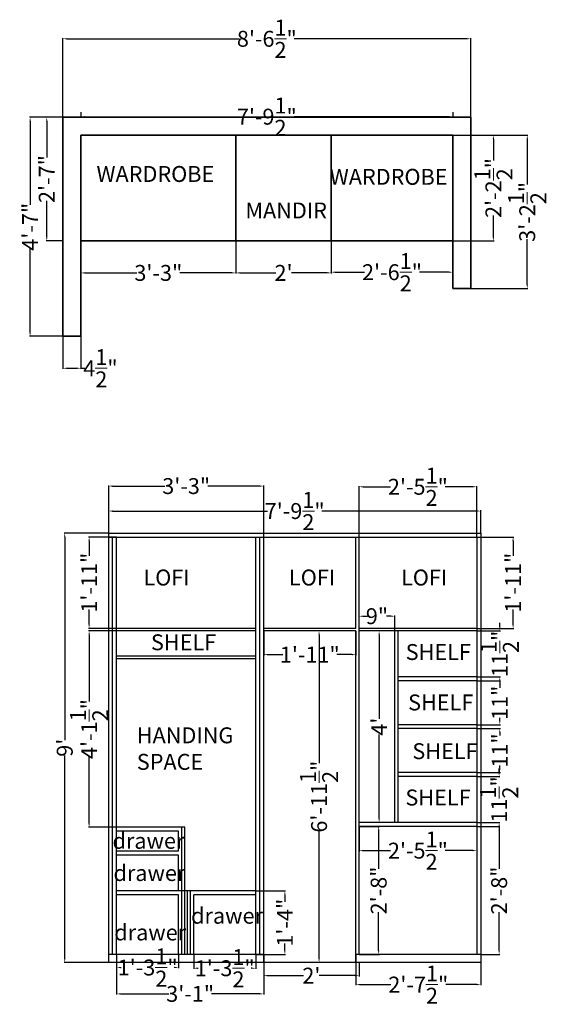
# Model space of a CAD drawing. Units: inches. Extents: x 198 to 331, y 201 to 449.
import ezdxf

# ---------------------------------------------------------------- set-up
doc = ezdxf.new("R2010")
doc.units = ezdxf.units.IN
doc.header["$MEASUREMENT"] = 0
for name, color, linetype, lineweight in [('A-ANNO-DIMS', 2, 'Continuous', 18), ('A-ANNO-TEXT', 3, 'Continuous', 18), ('A-ELEV', 7, 'Continuous', 25), ('A-FURN', 7, 'Continuous', 35)]:
    doc.layers.add(name, color=color, linetype=linetype, lineweight=lineweight)
doc.styles.get("Standard").update_dxf_attribs({"font": 'arial.ttf'})
doc.dimstyles.get("Standard").update_dxf_attribs({"dimtxt": 4, "dimasz": 1, "dimexe": 0.18, "dimexo": 0.0625, "dimgap": 0.09, "dimtad": 0, "dimdec": 1, "dimzin": 0, "dimdsep": 46, "dimlunit": 4, "dimtxsty": 'Standard', "dimcen": 0.09, "dimadec": 0, "dimazin": 0, "dimtfac": 1, "dimtdec": 1, "dimtofl": 0, "dimtmove": 0, "dimatfit": 3, "dimfxl": 1, "dimtolj": 1, "dimtzin": 0, "dimarcsym": 0})

# ---------------------------------------------------------------- blocks, each defined once
blk = doc.blocks.new('*D1')
at = {"layer": 'A-ANNO-DIMS', "color": 0, "lineweight": -2, "transparency": 16777216}
for p, q in [((307.47, 419.65), (317.79, 419.65)), ((317.61, 418.65), (317.61, 413.25)), ((317.61, 394.05), (317.61, 399.45)), ((307.47, 393.05), (317.79, 393.05))]:
    blk.add_line(p, q, dxfattribs=at)
at = {"layer": 'A-ANNO-DIMS', "color": 0, "transparency": 16777216}
for points in [[(317.44, 418.65), (317.77, 418.65), (317.61, 419.65)], [(317.44, 394.05), (317.77, 394.05), (317.61, 393.05)]]:
    blk.add_solid(points, dxfattribs=at)
at = {"layer": 'Defpoints', "color": 0, "transparency": 16777216}
for p in [(307.4, 419.65), (317.61, 419.65), (307.4, 393.05)]:
    blk.add_point(p, dxfattribs=at)
at = {"layer": 'A-ANNO-DIMS', "color": 0, "transparency": 16777216, "insert": (317.61, 406.35), "char_height": 4, "attachment_point": 5, "rotation": 90}
blk.add_mtext('\\A1;2\'-2{\\H1x;\\S1/2;}"', dxfattribs=at)
blk = doc.blocks.new('*D2')
at = {"layer": 'A-ANNO-DIMS', "color": 0, "lineweight": -2, "transparency": 16777216}
for p, q in [((276.8, 392.99), (276.8, 385)), ((307.4, 392.99), (307.4, 385)), ((277.8, 385.18), (285.21, 385.18)), ((306.4, 385.18), (299, 385.18))]:
    blk.add_line(p, q, dxfattribs=at)
at = {"layer": 'A-ANNO-DIMS', "color": 0, "transparency": 16777216}
for points in [[(277.8, 385.35), (277.8, 385.02), (276.8, 385.18)], [(306.4, 385.35), (306.4, 385.02), (307.4, 385.18)]]:
    blk.add_solid(points, dxfattribs=at)
at = {"layer": 'Defpoints', "color": 0, "transparency": 16777216}
for p in [(276.8, 393.05), (307.4, 393.05), (307.4, 385.18)]:
    blk.add_point(p, dxfattribs=at)
at = {"layer": 'A-ANNO-DIMS', "color": 0, "transparency": 16777216, "insert": (292.1, 385.18), "char_height": 4, "attachment_point": 5}
blk.add_mtext('\\A1;2\'-6{\\H1x;\\S1/2;}"', dxfattribs=at)
blk = doc.blocks.new('*D3')
at = {"layer": 'A-ANNO-DIMS', "color": 0, "lineweight": -2, "transparency": 16777216}
for p, q in [((252.8, 392.99), (252.8, 384.82)), ((276.8, 392.99), (276.8, 384.82)), ((253.8, 385), (262.84, 385)), ((275.8, 385), (266.77, 385))]:
    blk.add_line(p, q, dxfattribs=at)
at = {"layer": 'A-ANNO-DIMS', "color": 0, "transparency": 16777216}
for points in [[(253.8, 385.17), (253.8, 384.84), (252.8, 385)], [(275.8, 385.17), (275.8, 384.84), (276.8, 385)]]:
    blk.add_solid(points, dxfattribs=at)
at = {"layer": 'Defpoints', "color": 0, "transparency": 16777216}
for p in [(252.8, 393.05), (276.8, 393.05), (276.8, 385)]:
    blk.add_point(p, dxfattribs=at)
at = {"layer": 'A-ANNO-DIMS', "color": 0, "transparency": 16777216, "insert": (264.8, 385), "char_height": 4, "attachment_point": 5}
blk.add_mtext("\\A1;2'", dxfattribs=at)
blk = doc.blocks.new('*D4')
at = {"layer": 'A-ANNO-DIMS', "color": 0, "lineweight": -2, "transparency": 16777216}
for p, q in [((213.8, 392.99), (213.8, 384.82)), ((252.8, 392.99), (252.8, 384.82)), ((214.8, 385), (227.9, 385)), ((251.8, 385), (238.71, 385))]:
    blk.add_line(p, q, dxfattribs=at)
at = {"layer": 'A-ANNO-DIMS', "color": 0, "transparency": 16777216}
for points in [[(214.8, 385.17), (214.8, 384.84), (213.8, 385)], [(251.8, 385.17), (251.8, 384.84), (252.8, 385)]]:
    blk.add_solid(points, dxfattribs=at)
at = {"layer": 'Defpoints', "color": 0, "transparency": 16777216}
for p in [(213.8, 393.05), (252.8, 393.05), (252.8, 385)]:
    blk.add_point(p, dxfattribs=at)
at = {"layer": 'A-ANNO-DIMS', "color": 0, "transparency": 16777216, "insert": (233.3, 385), "char_height": 4, "attachment_point": 5}
blk.add_mtext('\\A1;3\'-3"', dxfattribs=at)
blk = doc.blocks.new('*D5')
at = {"layer": 'A-ANNO-DIMS', "color": 0, "lineweight": -2, "transparency": 16777216}
for p, q in [((213.8, 425.45), (213.8, 424.11)), ((214.8, 424.29), (253.76, 424.29)), ((306.4, 424.29), (267.45, 424.29)), ((307.4, 425.45), (307.4, 424.11))]:
    blk.add_line(p, q, dxfattribs=at)
at = {"layer": 'A-ANNO-DIMS', "color": 0, "transparency": 16777216}
for points in [[(214.8, 424.46), (214.8, 424.13), (213.8, 424.29)], [(306.4, 424.46), (306.4, 424.13), (307.4, 424.29)]]:
    blk.add_solid(points, dxfattribs=at)
at = {"layer": 'Defpoints', "color": 0, "transparency": 16777216}
for p in [(213.8, 425.51), (307.4, 425.51), (307.4, 424.29)]:
    blk.add_point(p, dxfattribs=at)
at = {"layer": 'A-ANNO-DIMS', "color": 0, "transparency": 16777216, "insert": (260.6, 424.29), "char_height": 4, "attachment_point": 5}
blk.add_mtext('\\A1;7\'-9{\\H1x;\\S1/2;}"', dxfattribs=at)
blk = doc.blocks.new('*D6')
at = {"layer": 'A-ANNO-DIMS', "color": 0, "lineweight": -2, "transparency": 16777216}
for p, q in [((222.81, 213.52), (222.81, 203.5)), ((259.81, 213.52), (259.81, 203.5)), ((223.81, 203.68), (235.91, 203.68)), ((258.81, 203.68), (246.72, 203.68))]:
    blk.add_line(p, q, dxfattribs=at)
at = {"layer": 'A-ANNO-DIMS', "color": 0, "transparency": 16777216}
for points in [[(223.81, 203.84), (223.81, 203.51), (222.81, 203.68)], [(258.81, 203.84), (258.81, 203.51), (259.81, 203.68)]]:
    blk.add_solid(points, dxfattribs=at)
at = {"layer": 'Defpoints', "color": 0, "transparency": 16777216}
for p in [(222.81, 213.58), (259.81, 213.58), (259.81, 203.68)]:
    blk.add_point(p, dxfattribs=at)
at = {"layer": 'A-ANNO-DIMS', "color": 0, "transparency": 16777216, "insert": (241.31, 203.68), "char_height": 4, "attachment_point": 5}
blk.add_mtext('\\A1;3\'-1"', dxfattribs=at)
blk = doc.blocks.new('*D7')
at = {"layer": 'A-ANNO-DIMS', "color": 0, "lineweight": -2, "transparency": 16777216}
for p, q in [((313.47, 318.58), (322.74, 318.58)), ((322.56, 317.58), (322.56, 313.85)), ((322.56, 296.58), (322.56, 300.31)), ((313.47, 295.58), (322.74, 295.58))]:
    blk.add_line(p, q, dxfattribs=at)
at = {"layer": 'A-ANNO-DIMS', "color": 0, "transparency": 16777216}
for points in [[(322.39, 317.58), (322.72, 317.58), (322.56, 318.58)], [(322.39, 296.58), (322.72, 296.58), (322.56, 295.58)]]:
    blk.add_solid(points, dxfattribs=at)
at = {"layer": 'Defpoints', "color": 0, "transparency": 16777216}
for p in [(313.41, 318.58), (313.41, 295.58), (322.56, 295.58)]:
    blk.add_point(p, dxfattribs=at)
at = {"layer": 'A-ANNO-DIMS', "color": 0, "transparency": 16777216, "insert": (322.56, 307.08), "char_height": 4, "attachment_point": 5, "rotation": 90}
blk.add_mtext('\\A1;1\'-11"', dxfattribs=at)
blk = doc.blocks.new('*D8')
at = {"layer": 'A-ANNO-DIMS', "color": 0, "lineweight": -2, "transparency": 16777216}
for p, q in [((313.47, 245.78), (319.23, 245.78)), ((319.05, 244.78), (319.05, 235.12)), ((319.05, 214.58), (319.05, 224.24)), ((314.47, 213.58), (319.23, 213.58))]:
    blk.add_line(p, q, dxfattribs=at)
at = {"layer": 'A-ANNO-DIMS', "color": 0, "transparency": 16777216}
for points in [[(318.88, 244.78), (319.21, 244.78), (319.05, 245.78)], [(318.88, 214.58), (319.21, 214.58), (319.05, 213.58)]]:
    blk.add_solid(points, dxfattribs=at)
at = {"layer": 'Defpoints', "color": 0, "transparency": 16777216}
for p in [(313.41, 245.78), (319.05, 245.78), (314.41, 213.58)]:
    blk.add_point(p, dxfattribs=at)
at = {"layer": 'A-ANNO-DIMS', "color": 0, "transparency": 16777216, "insert": (319.05, 229.68), "char_height": 4, "attachment_point": 5, "rotation": 90}
blk.add_mtext('\\A1;2\'-8"', dxfattribs=at)
blk = doc.blocks.new('*D9')
at = {"layer": 'A-ANNO-DIMS', "color": 0, "lineweight": -2, "transparency": 16777216}
for p, q in [((319.05, 259.38), (319.05, 260.38)), ((313.47, 258.38), (319.23, 258.38)), ((313.47, 246.78), (319.23, 246.78)), ((319.05, 245.78), (319.05, 244.78))]:
    blk.add_line(p, q, dxfattribs=at)
at = {"layer": 'A-ANNO-DIMS', "color": 0, "transparency": 16777216}
for points in [[(318.88, 259.38), (319.21, 259.38), (319.05, 258.38)], [(318.88, 245.78), (319.21, 245.78), (319.05, 246.78)]]:
    blk.add_solid(points, dxfattribs=at)
at = {"layer": 'Defpoints', "color": 0, "transparency": 16777216}
for p in [(313.41, 258.38), (313.41, 246.78), (319.05, 246.78)]:
    blk.add_point(p, dxfattribs=at)
at = {"layer": 'A-ANNO-DIMS', "color": 0, "transparency": 16777216, "insert": (319.05, 252.58), "char_height": 4, "attachment_point": 5, "rotation": 90}
blk.add_mtext('\\A1;11{\\H1x;\\S1/2;}"', dxfattribs=at)
blk = doc.blocks.new('*D10')
at = {"layer": 'A-ANNO-DIMS', "color": 0, "lineweight": -2, "transparency": 16777216}
for p, q in [((313.47, 270.38), (319.39, 270.38)), ((319.21, 269.38), (319.21, 268.63)), ((319.21, 260.38), (319.21, 261.13)), ((313.47, 259.38), (319.39, 259.38))]:
    blk.add_line(p, q, dxfattribs=at)
at = {"layer": 'A-ANNO-DIMS', "color": 0, "transparency": 16777216}
for points in [[(319.05, 269.38), (319.38, 269.38), (319.21, 270.38)], [(319.05, 260.38), (319.38, 260.38), (319.21, 259.38)]]:
    blk.add_solid(points, dxfattribs=at)
at = {"layer": 'Defpoints', "color": 0, "transparency": 16777216}
for p in [(313.41, 270.38), (313.41, 259.38), (319.21, 259.38)]:
    blk.add_point(p, dxfattribs=at)
at = {"layer": 'A-ANNO-DIMS', "color": 0, "transparency": 16777216, "insert": (319.21, 264.88), "char_height": 4, "attachment_point": 5, "rotation": 90}
blk.add_mtext('\\A1;11"', dxfattribs=at)
blk = doc.blocks.new('*D11')
at = {"layer": 'A-ANNO-DIMS', "color": 0, "lineweight": -2, "transparency": 16777216}
for p, q in [((313.47, 282.38), (319.39, 282.38)), ((319.21, 281.38), (319.21, 280.63)), ((319.21, 272.38), (319.21, 273.13)), ((313.47, 271.38), (319.39, 271.38))]:
    blk.add_line(p, q, dxfattribs=at)
at = {"layer": 'A-ANNO-DIMS', "color": 0, "transparency": 16777216}
for points in [[(319.05, 281.38), (319.38, 281.38), (319.21, 282.38)], [(319.05, 272.38), (319.38, 272.38), (319.21, 271.38)]]:
    blk.add_solid(points, dxfattribs=at)
at = {"layer": 'Defpoints', "color": 0, "transparency": 16777216}
for p in [(313.41, 282.38), (313.41, 271.38), (319.21, 271.38)]:
    blk.add_point(p, dxfattribs=at)
at = {"layer": 'A-ANNO-DIMS', "color": 0, "transparency": 16777216, "insert": (319.21, 276.88), "char_height": 4, "attachment_point": 5, "rotation": 90}
blk.add_mtext('\\A1;11"', dxfattribs=at)
blk = doc.blocks.new('*D12')
at = {"layer": 'A-ANNO-DIMS', "color": 0, "lineweight": -2, "transparency": 16777216}
for p, q in [((313.47, 294.98), (319.39, 294.98)), ((319.21, 295.98), (319.21, 296.98)), ((313.47, 283.38), (319.39, 283.38)), ((319.21, 282.38), (319.21, 281.38))]:
    blk.add_line(p, q, dxfattribs=at)
at = {"layer": 'A-ANNO-DIMS', "color": 0, "transparency": 16777216}
for points in [[(319.05, 295.98), (319.38, 295.98), (319.21, 294.98)], [(319.05, 282.38), (319.38, 282.38), (319.21, 283.38)]]:
    blk.add_solid(points, dxfattribs=at)
at = {"layer": 'Defpoints', "color": 0, "transparency": 16777216}
for p in [(313.41, 294.98), (313.41, 283.38), (319.21, 283.38)]:
    blk.add_point(p, dxfattribs=at)
at = {"layer": 'A-ANNO-DIMS', "color": 0, "transparency": 16777216, "insert": (319.21, 289.18), "char_height": 4, "attachment_point": 5, "rotation": 90}
blk.add_mtext('\\A1;11{\\H1x;\\S1/2;}"', dxfattribs=at)
blk = doc.blocks.new('*D13')
at = {"layer": 'A-ANNO-DIMS', "color": 0, "lineweight": -2, "transparency": 16777216}
for p, q in [((283.01, 213.52), (283.01, 205.83)), ((314.41, 213.52), (314.41, 205.83)), ((284.01, 206.01), (291.81, 206.01)), ((313.41, 206.01), (305.61, 206.01))]:
    blk.add_line(p, q, dxfattribs=at)
at = {"layer": 'A-ANNO-DIMS', "color": 0, "transparency": 16777216}
for points in [[(284.01, 206.17), (284.01, 205.84), (283.01, 206.01)], [(313.41, 206.17), (313.41, 205.84), (314.41, 206.01)]]:
    blk.add_solid(points, dxfattribs=at)
at = {"layer": 'Defpoints', "color": 0, "transparency": 16777216}
for p in [(283.01, 213.58), (314.41, 213.58), (283.01, 206.01)]:
    blk.add_point(p, dxfattribs=at)
at = {"layer": 'A-ANNO-DIMS', "color": 0, "transparency": 16777216, "insert": (298.71, 206.01), "char_height": 4, "attachment_point": 5}
blk.add_mtext('\\A1;2\'-7{\\H1x;\\S1/2;}"', dxfattribs=at)
blk = doc.blocks.new('*D14')
at = {"layer": 'A-ANNO-DIMS', "color": 0, "lineweight": -2, "transparency": 16777216}
for p, q in [((259.81, 211.52), (259.81, 208.08)), ((283.81, 211.52), (283.81, 208.08)), ((260.81, 208.26), (269.85, 208.26)), ((282.81, 208.26), (273.78, 208.26))]:
    blk.add_line(p, q, dxfattribs=at)
at = {"layer": 'A-ANNO-DIMS', "color": 0, "transparency": 16777216}
for points in [[(260.81, 208.43), (260.81, 208.09), (259.81, 208.26)], [(282.81, 208.43), (282.81, 208.09), (283.81, 208.26)]]:
    blk.add_solid(points, dxfattribs=at)
at = {"layer": 'Defpoints', "color": 0, "transparency": 16777216}
for p in [(259.81, 211.58), (283.81, 211.58), (283.81, 208.26)]:
    blk.add_point(p, dxfattribs=at)
at = {"layer": 'A-ANNO-DIMS', "color": 0, "transparency": 16777216, "insert": (271.81, 208.26), "char_height": 4, "attachment_point": 5}
blk.add_mtext("\\A1;2'", dxfattribs=at)
blk = doc.blocks.new('*D15')
at = {"layer": 'A-ANNO-DIMS', "color": 0, "lineweight": -2, "transparency": 16777216}
for p, q in [((222.81, 213.52), (222.81, 210.13)), ((238.41, 213.52), (238.41, 210.13)), ((223.81, 210.31), (223.93, 210.31)), ((237.41, 210.31), (237.29, 210.31))]:
    blk.add_line(p, q, dxfattribs=at)
at = {"layer": 'A-ANNO-DIMS', "color": 0, "transparency": 16777216}
for points in [[(223.81, 210.47), (223.81, 210.14), (222.81, 210.31)], [(237.41, 210.47), (237.41, 210.14), (238.41, 210.31)]]:
    blk.add_solid(points, dxfattribs=at)
at = {"layer": 'Defpoints', "color": 0, "transparency": 16777216}
for p in [(222.81, 213.58), (238.41, 213.58), (222.81, 210.31)]:
    blk.add_point(p, dxfattribs=at)
at = {"layer": 'A-ANNO-DIMS', "color": 0, "transparency": 16777216, "insert": (230.61, 210.31), "char_height": 4, "attachment_point": 5}
blk.add_mtext('\\A1;1\'-3{\\H1x;\\S1/2;}"', dxfattribs=at)
blk = doc.blocks.new('*D16')
at = {"layer": 'A-ANNO-DIMS', "color": 0, "lineweight": -2, "transparency": 16777216}
for p, q in [((242.21, 213.52), (242.21, 209.95)), ((257.81, 213.52), (257.81, 209.95)), ((243.21, 210.13), (243.33, 210.13)), ((256.81, 210.13), (256.69, 210.13))]:
    blk.add_line(p, q, dxfattribs=at)
at = {"layer": 'A-ANNO-DIMS', "color": 0, "transparency": 16777216}
for points in [[(243.21, 210.29), (243.21, 209.96), (242.21, 210.13)], [(256.81, 210.29), (256.81, 209.96), (257.81, 210.13)]]:
    blk.add_solid(points, dxfattribs=at)
at = {"layer": 'Defpoints', "color": 0, "transparency": 16777216}
for p in [(242.21, 213.58), (257.81, 213.58), (257.81, 210.13)]:
    blk.add_point(p, dxfattribs=at)
at = {"layer": 'A-ANNO-DIMS', "color": 0, "transparency": 16777216, "insert": (250.01, 210.13), "char_height": 4, "attachment_point": 5}
blk.add_mtext('\\A1;1\'-3{\\H1x;\\S1/2;}"', dxfattribs=at)
blk = doc.blocks.new('*D17')
at = {"layer": 'A-ANNO-DIMS', "color": 0, "lineweight": -2, "transparency": 16777216}
for p, q in [((257.87, 229.58), (265.32, 229.58)), ((265.14, 228.58), (265.14, 226.8)), ((265.14, 214.58), (265.14, 216.36)), ((257.87, 213.58), (265.32, 213.58))]:
    blk.add_line(p, q, dxfattribs=at)
at = {"layer": 'A-ANNO-DIMS', "color": 0, "transparency": 16777216}
for points in [[(264.98, 228.58), (265.31, 228.58), (265.14, 229.58)], [(264.98, 214.58), (265.31, 214.58), (265.14, 213.58)]]:
    blk.add_solid(points, dxfattribs=at)
at = {"layer": 'Defpoints', "color": 0, "transparency": 16777216}
for p in [(257.81, 229.58), (257.81, 213.58), (265.14, 213.58)]:
    blk.add_point(p, dxfattribs=at)
at = {"layer": 'A-ANNO-DIMS', "color": 0, "transparency": 16777216, "insert": (265.14, 221.58), "char_height": 4, "attachment_point": 5, "rotation": 90}
blk.add_mtext('\\A1;1\'-4"', dxfattribs=at)
blk = doc.blocks.new('*D18')
at = {"layer": 'A-ANNO-DIMS', "color": 0, "lineweight": -2, "transparency": 16777216}
for p, q in [((222.75, 294.98), (215.71, 294.98)), ((215.89, 293.98), (215.89, 277.22)), ((215.89, 246.58), (215.89, 263.33)), ((222.75, 245.58), (215.71, 245.58))]:
    blk.add_line(p, q, dxfattribs=at)
at = {"layer": 'A-ANNO-DIMS', "color": 0, "transparency": 16777216}
for points in [[(215.72, 293.98), (216.05, 293.98), (215.89, 294.98)], [(215.72, 246.58), (216.05, 246.58), (215.89, 245.58)]]:
    blk.add_solid(points, dxfattribs=at)
at = {"layer": 'Defpoints', "color": 0, "transparency": 16777216}
for p in [(215.89, 294.98), (222.81, 294.98), (222.81, 245.58)]:
    blk.add_point(p, dxfattribs=at)
at = {"layer": 'A-ANNO-DIMS', "color": 0, "transparency": 16777216, "insert": (215.89, 270.28), "char_height": 4, "attachment_point": 5, "rotation": 90}
blk.add_mtext('\\A1;4\'-1{\\H1x;\\S1/2;}"', dxfattribs=at)
blk = doc.blocks.new('*D19')
at = {"layer": 'A-ANNO-DIMS', "color": 0, "lineweight": -2, "transparency": 16777216}
for p, q in [((222.75, 318.58), (215.71, 318.58)), ((215.89, 317.58), (215.89, 313.85)), ((215.89, 296.58), (215.89, 300.31)), ((222.75, 295.58), (215.71, 295.58))]:
    blk.add_line(p, q, dxfattribs=at)
at = {"layer": 'A-ANNO-DIMS', "color": 0, "transparency": 16777216}
for points in [[(215.72, 317.58), (216.05, 317.58), (215.89, 318.58)], [(215.72, 296.58), (216.05, 296.58), (215.89, 295.58)]]:
    blk.add_solid(points, dxfattribs=at)
at = {"layer": 'Defpoints', "color": 0, "transparency": 16777216}
for p in [(215.89, 318.58), (222.81, 318.58), (222.81, 295.58)]:
    blk.add_point(p, dxfattribs=at)
at = {"layer": 'A-ANNO-DIMS', "color": 0, "transparency": 16777216, "insert": (215.89, 307.08), "char_height": 4, "attachment_point": 5, "rotation": 90}
blk.add_mtext('\\A1;1\'-11"', dxfattribs=at)
blk = doc.blocks.new('*D20')
at = {"layer": 'A-ANNO-DIMS', "color": 0, "lineweight": -2, "transparency": 16777216}
for p, q in [((220.81, 319.64), (220.81, 325.29)), ((221.81, 325.11), (260.76, 325.11)), ((313.41, 325.11), (274.46, 325.11)), ((314.41, 319.64), (314.41, 325.29))]:
    blk.add_line(p, q, dxfattribs=at)
at = {"layer": 'A-ANNO-DIMS', "color": 0, "transparency": 16777216}
for points in [[(221.81, 325.28), (221.81, 324.95), (220.81, 325.11)], [(313.41, 325.28), (313.41, 324.95), (314.41, 325.11)]]:
    blk.add_solid(points, dxfattribs=at)
at = {"layer": 'Defpoints', "color": 0, "transparency": 16777216}
for p in [(314.41, 325.11), (220.81, 319.58), (314.41, 319.58)]:
    blk.add_point(p, dxfattribs=at)
at = {"layer": 'A-ANNO-DIMS', "color": 0, "transparency": 16777216, "insert": (267.61, 325.11), "char_height": 4, "attachment_point": 5}
blk.add_mtext('\\A1;7\'-9{\\H1x;\\S1/2;}"', dxfattribs=at)
blk = doc.blocks.new('*D21')
at = {"layer": 'A-ANNO-DIMS', "color": 0, "lineweight": -2, "transparency": 16777216}
for p, q in [((220.75, 319.58), (209.57, 319.58)), ((209.75, 318.58), (209.75, 267.51)), ((209.75, 212.58), (209.75, 263.65)), ((220.75, 211.58), (209.57, 211.58))]:
    blk.add_line(p, q, dxfattribs=at)
at = {"layer": 'A-ANNO-DIMS', "color": 0, "transparency": 16777216}
for points in [[(209.59, 318.58), (209.92, 318.58), (209.75, 319.58)], [(209.59, 212.58), (209.92, 212.58), (209.75, 211.58)]]:
    blk.add_solid(points, dxfattribs=at)
at = {"layer": 'Defpoints', "color": 0, "transparency": 16777216}
for p in [(209.75, 319.58), (220.81, 319.58), (220.81, 211.58)]:
    blk.add_point(p, dxfattribs=at)
at = {"layer": 'A-ANNO-DIMS', "color": 0, "transparency": 16777216, "insert": (209.75, 265.58), "char_height": 4, "attachment_point": 5, "rotation": 90}
blk.add_mtext("\\A1;9'", dxfattribs=at)
blk = doc.blocks.new('*D22')
at = {"layer": 'A-ANNO-DIMS', "color": 0, "lineweight": -2, "transparency": 16777216}
for p, q in [((282.95, 294.98), (273.56, 294.98)), ((273.74, 293.98), (273.74, 261.71)), ((273.74, 212.58), (273.74, 244.85)), ((282.95, 211.58), (273.56, 211.58))]:
    blk.add_line(p, q, dxfattribs=at)
at = {"layer": 'A-ANNO-DIMS', "color": 0, "transparency": 16777216}
for points in [[(273.58, 293.98), (273.91, 293.98), (273.74, 294.98)], [(273.58, 212.58), (273.91, 212.58), (273.74, 211.58)]]:
    blk.add_solid(points, dxfattribs=at)
at = {"layer": 'Defpoints', "color": 0, "transparency": 16777216}
for p in [(273.74, 294.98), (283.01, 294.98), (283.01, 211.58)]:
    blk.add_point(p, dxfattribs=at)
at = {"layer": 'A-ANNO-DIMS', "color": 0, "transparency": 16777216, "insert": (273.74, 253.28), "char_height": 4, "attachment_point": 5, "rotation": 90}
blk.add_mtext('\\A1;6\'-11{\\H1x;\\S1/2;}"', dxfattribs=at)
blk = doc.blocks.new('*D23')
at = {"layer": 'A-ANNO-DIMS', "color": 0, "lineweight": -2, "transparency": 16777216}
for p, q in [((283.87, 245.78), (288.92, 245.78)), ((288.74, 244.78), (288.74, 235.12)), ((288.74, 214.58), (288.74, 224.24)), ((283.87, 213.58), (288.92, 213.58))]:
    blk.add_line(p, q, dxfattribs=at)
at = {"layer": 'A-ANNO-DIMS', "color": 0, "transparency": 16777216}
for points in [[(288.58, 244.78), (288.91, 244.78), (288.74, 245.78)], [(288.58, 214.58), (288.91, 214.58), (288.74, 213.58)]]:
    blk.add_solid(points, dxfattribs=at)
at = {"layer": 'Defpoints', "color": 0, "transparency": 16777216}
for p in [(283.81, 245.78), (283.81, 213.58), (288.74, 213.58)]:
    blk.add_point(p, dxfattribs=at)
at = {"layer": 'A-ANNO-DIMS', "color": 0, "transparency": 16777216, "insert": (288.74, 229.68), "char_height": 4, "attachment_point": 5, "rotation": 90}
blk.add_mtext('\\A1;2\'-8"', dxfattribs=at)
blk = doc.blocks.new('*D24')
at = {"layer": 'A-ANNO-DIMS', "color": 0, "lineweight": -2, "transparency": 16777216}
for p, q in [((283.81, 245.72), (283.81, 239.52)), ((313.41, 245.72), (313.41, 239.52)), ((284.81, 239.7), (291.71, 239.7)), ((312.41, 239.7), (305.51, 239.7))]:
    blk.add_line(p, q, dxfattribs=at)
at = {"layer": 'A-ANNO-DIMS', "color": 0, "transparency": 16777216}
for points in [[(284.81, 239.87), (284.81, 239.54), (283.81, 239.7)], [(312.41, 239.87), (312.41, 239.54), (313.41, 239.7)]]:
    blk.add_solid(points, dxfattribs=at)
at = {"layer": 'Defpoints', "color": 0, "transparency": 16777216}
for p in [(283.81, 245.78), (313.41, 245.78), (283.81, 239.7)]:
    blk.add_point(p, dxfattribs=at)
at = {"layer": 'A-ANNO-DIMS', "color": 0, "transparency": 16777216, "insert": (298.61, 239.7), "char_height": 4, "attachment_point": 5}
blk.add_mtext('\\A1;2\'-5{\\H1x;\\S1/2;}"', dxfattribs=at)
blk = doc.blocks.new('*D25')
at = {"layer": 'A-ANNO-DIMS', "color": 0, "lineweight": -2, "transparency": 16777216}
for p, q in [((259.81, 294.92), (259.81, 288.81)), ((283.01, 294.92), (283.01, 288.81)), ((260.81, 288.99), (264.64, 288.99)), ((282.01, 288.99), (278.18, 288.99))]:
    blk.add_line(p, q, dxfattribs=at)
at = {"layer": 'A-ANNO-DIMS', "color": 0, "transparency": 16777216}
for points in [[(260.81, 289.16), (260.81, 288.83), (259.81, 288.99)], [(282.01, 289.16), (282.01, 288.83), (283.01, 288.99)]]:
    blk.add_solid(points, dxfattribs=at)
at = {"layer": 'Defpoints', "color": 0, "transparency": 16777216}
for p in [(259.81, 294.98), (283.01, 294.98), (259.81, 288.99)]:
    blk.add_point(p, dxfattribs=at)
at = {"layer": 'A-ANNO-DIMS', "color": 0, "transparency": 16777216, "insert": (271.41, 288.99), "char_height": 4, "attachment_point": 5}
blk.add_mtext('\\A1;1\'-11"', dxfattribs=at)
blk = doc.blocks.new('*D26')
at = {"layer": 'A-ANNO-DIMS', "color": 0, "lineweight": -2, "transparency": 16777216}
for p, q in [((283.81, 295.04), (283.81, 298.84)), ((284.81, 298.66), (285.92, 298.66)), ((291.81, 298.66), (290.7, 298.66)), ((292.81, 295.04), (292.81, 298.84))]:
    blk.add_line(p, q, dxfattribs=at)
at = {"layer": 'A-ANNO-DIMS', "color": 0, "transparency": 16777216}
for points in [[(284.81, 298.83), (284.81, 298.49), (283.81, 298.66)], [(291.81, 298.83), (291.81, 298.49), (292.81, 298.66)]]:
    blk.add_solid(points, dxfattribs=at)
at = {"layer": 'Defpoints', "color": 0, "transparency": 16777216}
for p in [(292.81, 298.66), (283.81, 294.98), (292.81, 294.98)]:
    blk.add_point(p, dxfattribs=at)
at = {"layer": 'A-ANNO-DIMS', "color": 0, "transparency": 16777216, "insert": (288.31, 298.66), "char_height": 4, "attachment_point": 5}
blk.add_mtext('\\A1;9"', dxfattribs=at)
blk = doc.blocks.new('*D27')
at = {"layer": 'A-ANNO-DIMS', "color": 0, "lineweight": -2, "transparency": 16777216}
for p, q in [((292.75, 294.98), (288.68, 294.98)), ((288.86, 293.98), (288.86, 272.89)), ((288.86, 247.78), (288.86, 268.87)), ((292.75, 246.78), (288.68, 246.78))]:
    blk.add_line(p, q, dxfattribs=at)
at = {"layer": 'A-ANNO-DIMS', "color": 0, "transparency": 16777216}
for points in [[(288.7, 293.98), (289.03, 293.98), (288.86, 294.98)], [(288.7, 247.78), (289.03, 247.78), (288.86, 246.78)]]:
    blk.add_solid(points, dxfattribs=at)
at = {"layer": 'Defpoints', "color": 0, "transparency": 16777216}
for p in [(288.86, 294.98), (292.81, 294.98), (292.81, 246.78)]:
    blk.add_point(p, dxfattribs=at)
at = {"layer": 'A-ANNO-DIMS', "color": 0, "transparency": 16777216, "insert": (288.86, 270.88), "char_height": 4, "attachment_point": 5, "rotation": 90}
blk.add_mtext("\\A1;4'", dxfattribs=at)
blk = doc.blocks.new('*D28')
at = {"layer": 'A-ANNO-DIMS', "color": 0, "lineweight": -2, "transparency": 16777216}
for p, q in [((283.81, 318.64), (283.81, 331.39)), ((284.81, 331.21), (291.71, 331.21)), ((312.41, 331.21), (305.51, 331.21)), ((313.41, 318.64), (313.41, 331.39))]:
    blk.add_line(p, q, dxfattribs=at)
at = {"layer": 'A-ANNO-DIMS', "color": 0, "transparency": 16777216}
for points in [[(284.81, 331.37), (284.81, 331.04), (283.81, 331.21)], [(312.41, 331.37), (312.41, 331.04), (313.41, 331.21)]]:
    blk.add_solid(points, dxfattribs=at)
at = {"layer": 'Defpoints', "color": 0, "transparency": 16777216}
for p in [(283.81, 331.21), (283.81, 318.58), (313.41, 318.58)]:
    blk.add_point(p, dxfattribs=at)
at = {"layer": 'A-ANNO-DIMS', "color": 0, "transparency": 16777216, "insert": (298.61, 331.21), "char_height": 4, "attachment_point": 5}
blk.add_mtext('\\A1;2\'-5{\\H1x;\\S1/2;}"', dxfattribs=at)
blk = doc.blocks.new('*D29')
at = {"layer": 'A-ANNO-DIMS', "color": 0, "lineweight": -2, "transparency": 16777216}
for p, q in [((220.81, 318.64), (220.81, 331.57)), ((221.81, 331.39), (234.91, 331.39)), ((258.81, 331.39), (245.72, 331.39)), ((259.81, 318.64), (259.81, 331.57))]:
    blk.add_line(p, q, dxfattribs=at)
at = {"layer": 'A-ANNO-DIMS', "color": 0, "transparency": 16777216}
for points in [[(221.81, 331.55), (221.81, 331.22), (220.81, 331.39)], [(258.81, 331.55), (258.81, 331.22), (259.81, 331.39)]]:
    blk.add_solid(points, dxfattribs=at)
at = {"layer": 'Defpoints', "color": 0, "transparency": 16777216}
for p in [(259.81, 331.39), (220.81, 318.58), (259.81, 318.58)]:
    blk.add_point(p, dxfattribs=at)
at = {"layer": 'A-ANNO-DIMS', "color": 0, "transparency": 16777216, "insert": (240.31, 331.39), "char_height": 4, "attachment_point": 5}
blk.add_mtext('\\A1;3\'-3"', dxfattribs=at)
blk = doc.blocks.new('*D30')
at = {"layer": 'A-ANNO-DIMS', "color": 0, "lineweight": -2, "transparency": 16777216}
for p, q in [((209.3, 424.21), (209.3, 444.06)), ((210.3, 443.88), (253.74, 443.88)), ((310.9, 443.88), (267.47, 443.88)), ((311.9, 424.21), (311.9, 444.06))]:
    blk.add_line(p, q, dxfattribs=at)
at = {"layer": 'A-ANNO-DIMS', "color": 0, "transparency": 16777216}
for points in [[(210.3, 444.05), (210.3, 443.72), (209.3, 443.88)], [(310.9, 444.05), (310.9, 443.72), (311.9, 443.88)]]:
    blk.add_solid(points, dxfattribs=at)
at = {"layer": 'Defpoints', "color": 0, "transparency": 16777216}
for p in [(311.9, 443.88), (209.3, 424.15), (311.9, 424.15)]:
    blk.add_point(p, dxfattribs=at)
at = {"layer": 'A-ANNO-DIMS', "color": 0, "transparency": 16777216, "insert": (260.6, 443.88), "char_height": 4, "attachment_point": 5}
blk.add_mtext('\\A1;8\'-6{\\H1x;\\S1/2;}"', dxfattribs=at)
blk = doc.blocks.new('*D31')
at = {"layer": 'A-ANNO-DIMS', "color": 0, "lineweight": -2, "transparency": 16777216}
for p, q in [((209.24, 424.15), (205.05, 424.15)), ((205.23, 423.15), (205.23, 414.04)), ((205.23, 394.05), (205.23, 403.16)), ((209.24, 393.05), (205.05, 393.05))]:
    blk.add_line(p, q, dxfattribs=at)
at = {"layer": 'A-ANNO-DIMS', "color": 0, "transparency": 16777216}
for points in [[(205.07, 423.15), (205.4, 423.15), (205.23, 424.15)], [(205.07, 394.05), (205.4, 394.05), (205.23, 393.05)]]:
    blk.add_solid(points, dxfattribs=at)
at = {"layer": 'Defpoints', "color": 0, "transparency": 16777216}
for p in [(209.3, 424.15), (205.23, 393.05), (209.3, 393.05)]:
    blk.add_point(p, dxfattribs=at)
at = {"layer": 'A-ANNO-DIMS', "color": 0, "transparency": 16777216, "insert": (205.23, 408.6), "char_height": 4, "attachment_point": 5, "rotation": 90}
blk.add_mtext('\\A1;2\'-7"', dxfattribs=at)
blk = doc.blocks.new('*D32')
at = {"layer": 'A-ANNO-DIMS', "color": 0, "lineweight": -2, "transparency": 16777216}
for p, q in [((209.24, 424.15), (200.86, 424.15)), ((201.04, 423.15), (201.04, 402.09)), ((201.04, 370.05), (201.04, 391.11)), ((209.24, 369.05), (200.86, 369.05))]:
    blk.add_line(p, q, dxfattribs=at)
at = {"layer": 'A-ANNO-DIMS', "color": 0, "transparency": 16777216}
for points in [[(200.87, 423.15), (201.21, 423.15), (201.04, 424.15)], [(200.87, 370.05), (201.21, 370.05), (201.04, 369.05)]]:
    blk.add_solid(points, dxfattribs=at)
at = {"layer": 'Defpoints', "color": 0, "transparency": 16777216}
for p in [(209.3, 424.15), (201.04, 369.05), (209.3, 369.05)]:
    blk.add_point(p, dxfattribs=at)
at = {"layer": 'A-ANNO-DIMS', "color": 0, "transparency": 16777216, "insert": (201.04, 396.6), "char_height": 4, "attachment_point": 5, "rotation": 90}
blk.add_mtext('\\A1;4\'-7"', dxfattribs=at)
blk = doc.blocks.new('*D33')
at = {"layer": 'A-ANNO-DIMS', "color": 0, "lineweight": -2, "transparency": 16777216}
for p, q in [((209.3, 368.99), (209.3, 360.84)), ((213.8, 368.99), (213.8, 360.84)), ((210.3, 361.02), (212.8, 361.02)), ((213.8, 361.02), (214.8, 361.02))]:
    blk.add_line(p, q, dxfattribs=at)
at = {"layer": 'A-ANNO-DIMS', "color": 0, "transparency": 16777216}
for points in [[(210.3, 361.18), (210.3, 360.85), (209.3, 361.02)], [(212.8, 361.18), (212.8, 360.85), (213.8, 361.02)]]:
    blk.add_solid(points, dxfattribs=at)
at = {"layer": 'Defpoints', "color": 0, "transparency": 16777216}
for p in [(209.3, 369.05), (213.8, 369.05), (213.8, 361.02)]:
    blk.add_point(p, dxfattribs=at)
at = {"layer": 'A-ANNO-DIMS', "color": 0, "transparency": 16777216, "insert": (218.73, 361.02), "char_height": 4, "attachment_point": 5}
blk.add_mtext('\\A1;4{\\H1x;\\S1/2;}"', dxfattribs=at)
blk = doc.blocks.new('*D34')
at = {"layer": 'A-ANNO-DIMS', "color": 0, "lineweight": -2, "transparency": 16777216}
for p, q in [((311.97, 419.65), (326.3, 419.65)), ((326.12, 418.65), (326.12, 407.21)), ((326.12, 382.05), (326.12, 393.48)), ((311.97, 381.05), (326.3, 381.05))]:
    blk.add_line(p, q, dxfattribs=at)
at = {"layer": 'A-ANNO-DIMS', "color": 0, "transparency": 16777216}
for points in [[(325.96, 418.65), (326.29, 418.65), (326.12, 419.65)], [(325.96, 382.05), (326.29, 382.05), (326.12, 381.05)]]:
    blk.add_solid(points, dxfattribs=at)
at = {"layer": 'Defpoints', "color": 0, "transparency": 16777216}
for p in [(311.9, 419.65), (311.9, 381.05), (326.12, 381.05)]:
    blk.add_point(p, dxfattribs=at)
at = {"layer": 'A-ANNO-DIMS', "color": 0, "transparency": 16777216, "insert": (326.12, 400.35), "char_height": 4, "attachment_point": 5, "rotation": 90}
blk.add_mtext('\\A1;3\'-2{\\H1x;\\S1/2;}"', dxfattribs=at)

msp = doc.modelspace()

# ---------------------------------------------------------------- linework, layer by layer
at = {"layer": 'A-ELEV'}
for p, q in [((220.81, 211.58), (220.81, 319.58)), ((220.81, 319.58), (314.41, 319.58)), ((314.41, 319.58), (314.41, 211.58)), ((220.81, 318.58), (314.41, 318.58)), ((221.81, 213.58), (221.81, 318.58)), ((222.81, 213.58), (222.81, 318.58)), ((257.81, 213.58), (257.81, 318.58)), ((258.81, 213.58), (258.81, 318.58)), ((259.81, 211.58), (259.81, 318.58)), ((283.01, 295.58), (283.01, 318.58)), ((283.81, 295.58), (283.81, 318.58)), ((313.41, 318.58), (313.41, 213.58)), ((257.81, 295.58), (222.81, 295.58)), ((257.81, 294.98), (222.81, 294.98)), ((283.01, 295.58), (259.81, 295.58)), ((283.01, 294.98), (259.81, 294.98)), ((283.01, 211.58), (283.01, 294.98)), ((313.41, 295.58), (283.81, 295.58)), ((283.81, 213.58), (283.81, 294.98)), ((313.41, 294.98), (283.81, 294.98)), ((292.81, 246.78), (292.81, 294.98)), ((293.61, 246.78), (293.61, 294.98)), ((257.81, 288.58), (222.81, 288.58)), ((257.81, 287.98), (222.81, 287.98)), ((313.41, 283.38), (293.61, 283.38)), ((313.41, 282.38), (293.61, 282.38)), ((313.41, 271.38), (293.61, 271.38)), ((313.41, 270.38), (293.61, 270.38)), ((313.41, 259.38), (293.61, 259.38)), ((313.41, 258.38), (293.61, 258.38)), ((240.01, 245.58), (222.81, 245.58)), ((239.21, 213.58), (239.21, 245.58)), ((240.01, 213.58), (240.01, 245.58)), ((313.41, 246.78), (283.81, 246.78)), ((313.41, 245.78), (283.81, 245.78)), ((238.41, 244.58), (222.81, 244.58)), ((238.41, 239.58), (238.41, 244.58)), ((238.41, 239.58), (222.81, 239.58)), ((238.41, 238.58), (222.81, 238.58)), ((238.41, 229.58), (238.41, 238.58)), ((257.81, 229.58), (222.81, 229.58)), ((238.41, 228.58), (222.81, 228.58)), ((238.41, 213.58), (238.41, 228.58)), ((240.61, 213.58), (240.61, 229.58)), ((241.41, 213.58), (241.41, 229.58)), ((242.21, 213.58), (242.21, 228.58)), ((257.81, 228.58), (242.21, 228.58)), ((259.81, 213.58), (220.81, 213.58)), ((314.41, 213.58), (283.01, 213.58)), ((314.41, 211.58), (220.81, 211.58))]:
    msp.add_line(p, q, dxfattribs=at)
at = {"layer": 'A-FURN'}
for p, q in [((209.3, 424.15), (209.3, 393.05)), ((209.3, 424.15), (311.9, 424.15)), ((311.9, 393.05), (311.9, 424.15)), ((213.8, 419.65), (307.4, 419.65)), ((213.8, 419.65), (213.8, 393.05)), ((252.8, 393.05), (252.8, 419.65)), ((276.8, 393.05), (276.8, 419.65)), ((307.4, 393.05), (307.4, 419.65)), ((209.3, 393.05), (209.3, 369.05)), ((213.8, 393.05), (307.4, 393.05)), ((213.8, 369.05), (213.8, 393.05)), ((307.4, 381.05), (307.4, 393.05)), ((311.9, 393.05), (311.9, 381.05)), ((311.9, 381.05), (307.4, 381.05)), ((209.3, 369.05), (213.8, 369.05))]:
    msp.add_line(p, q, dxfattribs=at)

# ---------------------------------------------------------------- texts
at = {"layer": 'A-ANNO-TEXT', "char_height": 4, "attachment_point": 1}
for s, width, insert in [('WARDROBE', 30.7907, (217.74, 411.88)), ('WARDROBE', 30.7907, (276.43, 411.16)), ('\\pxqc;MANDIR', 30.1276, (250.41, 402.7)), ('LOFI', 22.1019, (229.55, 310.39)), ('LOFI', 22.1019, (266.17, 310.39)), ('LOFI', 22.1019, (294.37, 310.39)), ('\\pxqc;SHELF', 30.5801, (224.36, 294.1)), ('\\pxqc;SHELF', 30.5801, (288.46, 291.65)), ('\\pxqc;SHELF', 30.5801, (289.06, 278.97)), ('HANDING\\PSPACE', 26.9717, (227.88, 270.7)), ('\\pxqc;SHELF', 30.5801, (290.13, 266.72)), ('\\pxqc;SHELF', 30.5801, (288.38, 255.06)), ('\\pxqc;drawer', 13.6234, (224, 244.16)), ('\\pxqc;drawer', 13.6234, (224.24, 236.07)), ('\\pxqc;drawer', 13.6234, (243.77, 225.33)), ('\\pxqc;drawer', 13.6234, (224.44, 221.12))]:
    msp.add_mtext_dynamic_manual_height_columns(s, width=width, gutter_width=20, heights=[0], dxfattribs=dict(at, insert=insert))

# ---------------------------------------------------------------- dimensions: what is measured, and where the dimension line sits
at = {"layer": 'A-ANNO-DIMS'}
for base, p1, p2, picture, middle in [((311.9, 443.88), (209.3, 424.15), (311.9, 424.15), '*D30', (260.6, 443.88)), ((307.4, 424.29), (213.8, 425.51), (307.4, 425.51), '*D5', (260.6, 424.29)), ((252.8, 385), (213.8, 393.05), (252.8, 393.05), '*D4', (233.3, 385)), ((276.8, 385), (252.8, 393.05), (276.8, 393.05), '*D3', (264.8, 385)), ((307.4, 385.18), (276.8, 393.05), (307.4, 393.05), '*D2', (292.1, 385.18)), ((213.8, 361.02), (209.3, 369.05), (213.8, 369.05), '*D33', (218.73, 361.02)), ((283.81, 331.21), (313.41, 318.58), (283.81, 318.58), '*D28', (298.61, 331.21)), ((259.81, 331.39), (220.81, 318.58), (259.81, 318.58), '*D29', (240.31, 331.39)), ((314.41, 325.11), (220.81, 319.58), (314.41, 319.58), '*D20', (267.61, 325.11)), ((292.81, 298.66), (283.81, 294.98), (292.81, 294.98), '*D26', (288.31, 298.66)), ((259.81, 288.99), (283.01, 294.98), (259.81, 294.98), '*D25', (271.41, 288.99)), ((283.81, 239.7), (313.41, 245.78), (283.81, 245.78), '*D24', (298.61, 239.7)), ((222.81, 210.31), (238.41, 213.58), (222.81, 213.58), '*D15', (230.61, 210.31)), ((259.81, 203.68), (222.81, 213.58), (259.81, 213.58), '*D6', (241.31, 203.68)), ((257.81, 210.13), (242.21, 213.58), (257.81, 213.58), '*D16', (250.01, 210.13)), ((283.01, 206.01), (314.41, 213.58), (283.01, 213.58), '*D13', (298.71, 206.01)), ((283.81, 208.26), (259.81, 211.58), (283.81, 211.58), '*D14', (271.81, 208.26))]:
    dim = msp.add_linear_dim(base=base, p1=p1, p2=p2, dimstyle='Standard', override={"dimclrd": 0, "dimclre": 0, "dimclrt": 0}, dxfattribs=at)
    dim.commit()
    dim.dimension.update_dxf_attribs({"geometry": picture, "text_midpoint": middle})
for base, p1, p2, picture, middle in [((201.04, 369.05), (209.3, 424.15), (209.3, 369.05), '*D32', (201.04, 396.6)), ((205.23, 393.05), (209.3, 424.15), (209.3, 393.05), '*D31', (205.23, 408.6)), ((317.61, 419.65), (307.4, 393.05), (307.4, 419.65), '*D1', (317.61, 406.35)), ((326.12, 381.05), (311.9, 419.65), (311.9, 381.05), '*D34', (326.12, 400.35)), ((209.75, 319.58), (220.81, 211.58), (220.81, 319.58), '*D21', (209.75, 265.58)), ((215.89, 318.58), (222.81, 295.58), (222.81, 318.58), '*D19', (215.89, 307.08)), ((322.56, 295.58), (313.41, 318.58), (313.41, 295.58), '*D7', (322.56, 307.08)), ((319.21, 283.38), (313.41, 294.98), (313.41, 283.38), '*D12', (319.21, 289.18)), ((215.89, 294.98), (222.81, 245.58), (222.81, 294.98), '*D18', (215.89, 270.28)), ((273.74, 294.98), (283.01, 211.58), (283.01, 294.98), '*D22', (273.74, 253.28)), ((288.86, 294.98), (292.81, 246.78), (292.81, 294.98), '*D27', (288.86, 270.88)), ((319.21, 271.38), (313.41, 282.38), (313.41, 271.38), '*D11', (319.21, 276.88)), ((319.21, 259.38), (313.41, 270.38), (313.41, 259.38), '*D10', (319.21, 264.88)), ((319.05, 246.78), (313.41, 258.38), (313.41, 246.78), '*D9', (319.05, 252.58)), ((288.74, 213.58), (283.81, 245.78), (283.81, 213.58), '*D23', (288.74, 229.68)), ((319.05, 245.78), (314.41, 213.58), (313.41, 245.78), '*D8', (319.05, 229.68)), ((265.14, 213.58), (257.81, 229.58), (257.81, 213.58), '*D17', (265.14, 221.58))]:
    dim = msp.add_linear_dim(base=base, p1=p1, p2=p2, angle=90, dimstyle='Standard', override={"dimclrd": 0, "dimclre": 0, "dimclrt": 0}, dxfattribs=at)
    dim.commit()
    dim.dimension.update_dxf_attribs({"geometry": picture, "text_midpoint": middle})

doc.saveas('drawing.dxf')
